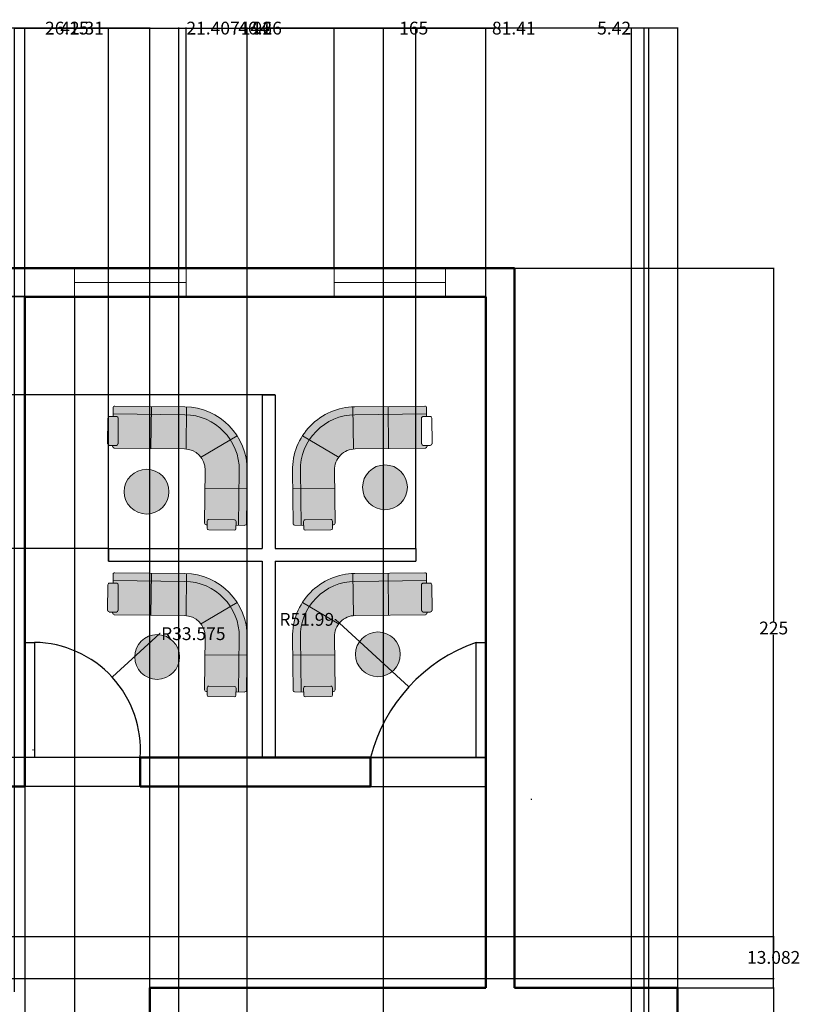
# Model space of a CAD drawing. Units: inches. Extents: x 1454 to 2136, y 626 to 1213.
# Tile 23 of 23: x 1887 to 2131, y 905 to 1213. Entities that reach past the tile are written whole.
import ezdxf

# ---------------------------------------------------------------- set-up
doc = ezdxf.new("R2010")
doc.units = ezdxf.units.IN
doc.header["$MEASUREMENT"] = 0
for name, color, linetype, lineweight in [('A-ANNO-DIMS', 2, 'Continuous', 18), ('A-DOOR', 3, 'Continuous', 25), ('A-FURN', 9, 'Continuous', 18), ('A-FURN-PATT', 252, 'Continuous', 13), ('A-FURN-PNLS', 8, 'Continuous', 25), ('A-GLAZ', 4, 'Continuous', 18), ('A-WALL', 7, 'Continuous', 50), ('sofa', 4, 'Continuous', 18)]:
    doc.layers.add(name, color=color, linetype=linetype, lineweight=lineweight)
doc.styles.get("Standard").update_dxf_attribs({"font": 'arial.ttf'})
doc.dimstyles.get("Standard").update_dxf_attribs({"dimtxt": 4, "dimasz": 0.18, "dimexe": 0.18, "dimexo": 0.0625, "dimgap": 0.09, "dimtad": 0, "dimtih": 1, "dimtoh": 1, "dimdec": 0, "dimrnd": 6, "dimzin": 0, "dimdsep": 46, "dimlunit": 3, "dimtxsty": 'Standard', "dimcen": 0.09, "dimadec": 0, "dimazin": 0, "dimtfac": 1, "dimtdec": 0, "dimtofl": 0, "dimtmove": 0, "dimatfit": 3, "dimfxl": 1, "dimtolj": 1, "dimtzin": 0, "dimarcsym": 0})

# ---------------------------------------------------------------- blocks, each defined once
blk = doc.blocks.new('A$C42183DBB')
for p, q in [((0.144, 1.661), (0.144, 1.562)), ((0.166, 1.682), (0.518, 1.682)), ((0.54, 1.661), (0.54, 1.562)), ((0, 1.592), (0, 0.864)), ((0.022, 1.614), (0.144, 1.614)), ((0.108, 1.614), (0.108, 0.864)), ((0.166, 1.541), (0.518, 1.541)), ((0.54, 1.614), (0.554, 1.614)), ((0.576, 1.592), (0.576, 0.864)), ((0, 1.11), (0.576, 1.11)), ((0.643, 0.69), (0.142, 0.389)), ((0.84, 0.576), (0.84, 0)), ((0.864, 0.576), (1.826, 0.576)), ((1.322, 0.576), (1.322, 0)), ((1.895, 0.54), (1.797, 0.54)), ((1.848, 0.54), (1.848, 0.554)), ((1.775, 0.166), (1.775, 0.518)), ((1.917, 0.166), (1.917, 0.518)), ((1.895, 0.144), (1.797, 0.144)), ((1.848, 0.022), (1.848, 0.144)), ((0.864, 0.108), (1.848, 0.108)), ((0.864, 0), (1.826, 0))]:
    blk.add_line(p, q)
for centre, radius, start, end in [((0.166, 1.661), 0.0216, 90, 180), ((0.518, 1.661), 0.0216, 0, 90), ((0.022, 1.592), 0.0216, 90, 180), ((0.166, 1.562), 0.0216, 180, 270), ((0.518, 1.562), 0.0216, 270, 0), ((0.554, 1.592), 0.0216, 0, 90), ((0.864, 0.864), 0.864, 180, 270), ((0.864, 0.864), 0.756, 180, 270), ((0.864, 0.864), 0.288, 180, 270), ((1.797, 0.518), 0.0216, 90, 180), ((1.826, 0.554), 0.0216, 0, 90), ((1.895, 0.518), 0.0216, 0, 90), ((1.797, 0.166), 0.0216, 180, 270), ((1.895, 0.166), 0.0216, 270, 0), ((1.826, 0.022), 0.0216, 270, 0)]:
    blk.add_arc(centre, radius, start, end)
blk = doc.blocks.new('WIN-34_84')
blk.add_line((34.84, 4.31), (0, 4.31))
blk.add_lwpolyline([(34.84, 0), (0, 0), (0, 9), (34.84, 9)], close=True)
blk = doc.blocks.new('DOOR-LEAF-36')
blk.add_lwpolyline([(-36, 3), (0, 3), (0, 0), (-36, 0)], close=True)
blk = doc.blocks.new('*D32')
at = {"layer": 'A-ANNO-DIMS', "color": 0, "lineweight": -2, "transparency": 16777216}
for p, q in [((1888.56, 1126.34), (1888.56, 1210.46)), ((1888.74, 1210.28), (1956.24, 1210.28)), ((2032.38, 1210.28), (1964.87, 1210.28)), ((2032.56, 1126.34), (2032.56, 1210.46))]:
    blk.add_line(p, q, dxfattribs=at)
at = {"layer": 'A-ANNO-DIMS', "color": 0, "transparency": 16777216}
for points in [[(1888.74, 1210.31), (1888.74, 1210.25), (1888.56, 1210.28)], [(2032.38, 1210.31), (2032.38, 1210.25), (2032.56, 1210.28)]]:
    blk.add_solid(points, dxfattribs=at)
at = {"layer": 'Defpoints', "color": 0, "transparency": 16777216}
for p in [(2032.56, 1210.28), (1888.56, 1126.28), (2032.56, 1126.28)]:
    blk.add_point(p, dxfattribs=at)
at = {"layer": 'A-ANNO-DIMS', "color": 0, "transparency": 16777216, "insert": (1960.56, 1210.28), "char_height": 4, "attachment_point": 5}
blk.add_mtext('\\A1;144', dxfattribs=at)
blk = doc.blocks.new('*D33')
at = {"layer": 'A-ANNO-DIMS', "color": 0, "lineweight": -2, "transparency": 16777216}
for p, q in [((2032.49, 1126.28), (1462.37, 1126.28)), ((1462.55, 1126.1), (1462.55, 1056.38)), ((1462.55, 982.46), (1462.55, 1052.18)), ((2032.49, 982.28), (1462.37, 982.28))]:
    blk.add_line(p, q, dxfattribs=at)
at = {"layer": 'A-ANNO-DIMS', "color": 0, "transparency": 16777216}
for points in [[(1462.52, 1126.1), (1462.58, 1126.1), (1462.55, 1126.28)], [(1462.52, 982.46), (1462.58, 982.46), (1462.55, 982.28)]]:
    blk.add_solid(points, dxfattribs=at)
at = {"layer": 'Defpoints', "color": 0, "transparency": 16777216}
for p in [(1462.55, 1126.28), (2032.56, 1126.28), (2032.56, 982.28)]:
    blk.add_point(p, dxfattribs=at)
at = {"layer": 'A-ANNO-DIMS', "color": 0, "transparency": 16777216, "insert": (1462.55, 1054.28), "char_height": 4, "attachment_point": 5}
blk.add_mtext('\\A1;144', dxfattribs=at)
blk = doc.blocks.new('*D34')
at = {"layer": 'A-ANNO-DIMS', "color": 0, "lineweight": -2, "transparency": 16777216}
for p, q in [((2041.62, 1135.28), (2122.74, 1135.28)), ((2122.56, 1135.1), (2122.56, 1024.91)), ((2122.56, 910.46), (2122.56, 1020.65)), ((2041.62, 910.28), (2122.74, 910.28))]:
    blk.add_line(p, q, dxfattribs=at)
at = {"layer": 'A-ANNO-DIMS', "color": 0, "transparency": 16777216}
for points in [[(2122.53, 1135.1), (2122.59, 1135.1), (2122.56, 1135.28)], [(2122.53, 910.46), (2122.59, 910.46), (2122.56, 910.28)]]:
    blk.add_solid(points, dxfattribs=at)
at = {"layer": 'Defpoints', "color": 0, "transparency": 16777216}
for p in [(2041.56, 1135.28), (2041.56, 910.28), (2122.56, 910.28)]:
    blk.add_point(p, dxfattribs=at)
at = {"layer": 'A-ANNO-DIMS', "color": 0, "transparency": 16777216, "insert": (2122.56, 1022.78), "char_height": 4, "attachment_point": 5}
blk.add_mtext('\\A1;225', dxfattribs=at)
blk = doc.blocks.new('*D35')
at = {"layer": 'A-ANNO-DIMS', "color": 0, "lineweight": -2, "transparency": 16777216}
for p, q in [((2092.62, 910.28), (2122.74, 910.28)), ((2122.56, 910.1), (2122.56, 808.91)), ((2122.56, 703.46), (2122.56, 804.65)), ((2092.62, 703.28), (2122.74, 703.28))]:
    blk.add_line(p, q, dxfattribs=at)
at = {"layer": 'A-ANNO-DIMS', "color": 0, "transparency": 16777216}
for points in [[(2122.53, 910.1), (2122.59, 910.1), (2122.56, 910.28)], [(2122.53, 703.46), (2122.59, 703.46), (2122.56, 703.28)]]:
    blk.add_solid(points, dxfattribs=at)
at = {"layer": 'Defpoints', "color": 0, "transparency": 16777216}
for p in [(2092.56, 910.28), (2092.56, 703.28), (2122.56, 703.28)]:
    blk.add_point(p, dxfattribs=at)
at = {"layer": 'A-ANNO-DIMS', "color": 0, "transparency": 16777216, "insert": (2122.56, 806.78), "char_height": 4, "attachment_point": 5}
blk.add_mtext('\\A1;207', dxfattribs=at)
blk = doc.blocks.new('*D36')
at = {"layer": 'A-ANNO-DIMS', "color": 0, "lineweight": -2, "transparency": 16777216}
for p, q in [((1927.56, 910.34), (1927.56, 1210.46)), ((1927.74, 1210.28), (2005.72, 1210.28)), ((2092.38, 1210.28), (2014.39, 1210.28)), ((2092.56, 910.34), (2092.56, 1210.46))]:
    blk.add_line(p, q, dxfattribs=at)
at = {"layer": 'A-ANNO-DIMS', "color": 0, "transparency": 16777216}
for points in [[(1927.74, 1210.31), (1927.74, 1210.25), (1927.56, 1210.28)], [(2092.38, 1210.31), (2092.38, 1210.25), (2092.56, 1210.28)]]:
    blk.add_solid(points, dxfattribs=at)
at = {"layer": 'Defpoints', "color": 0, "transparency": 16777216}
for p in [(2092.56, 1210.28), (1927.56, 910.28), (2092.56, 910.28)]:
    blk.add_point(p, dxfattribs=at)
at = {"layer": 'A-ANNO-DIMS', "color": 0, "transparency": 16777216, "insert": (2010.06, 1210.28), "char_height": 4, "attachment_point": 5}
blk.add_mtext('\\A1;165', dxfattribs=at)
blk = doc.blocks.new('*D37')
at = {"layer": 'A-ANNO-DIMS', "color": 0, "lineweight": -2, "transparency": 16777216}
for p, q in [((1774.56, 712.34), (1774.56, 1210.46)), ((1774.74, 1210.28), (1846.74, 1210.28)), ((1927.38, 1210.28), (1855.38, 1210.28)), ((1927.56, 712.34), (1927.56, 1210.46))]:
    blk.add_line(p, q, dxfattribs=at)
at = {"layer": 'A-ANNO-DIMS', "color": 0, "transparency": 16777216}
for points in [[(1774.74, 1210.31), (1774.74, 1210.25), (1774.56, 1210.28)], [(1927.38, 1210.31), (1927.38, 1210.25), (1927.56, 1210.28)]]:
    blk.add_solid(points, dxfattribs=at)
at = {"layer": 'Defpoints', "color": 0, "transparency": 16777216}
for p in [(1927.56, 1210.28), (1774.56, 712.28), (1927.56, 712.28)]:
    blk.add_point(p, dxfattribs=at)
at = {"layer": 'A-ANNO-DIMS', "color": 0, "transparency": 16777216, "insert": (1851.06, 1210.28), "char_height": 4, "attachment_point": 5}
blk.add_mtext('\\A1;153', dxfattribs=at)
blk = doc.blocks.new('*D47')
at = {"layer": 'A-ANNO-DIMS', "color": 0, "lineweight": -2, "transparency": 16777216}
for p, q in [((1885.25, 909.11), (1885.25, 1210.46)), ((1885.43, 1210.28), (1899.87, 1210.28)), ((1927.38, 1210.28), (1912.94, 1210.28)), ((1927.56, 910.34), (1927.56, 1210.46))]:
    blk.add_line(p, q, dxfattribs=at)
at = {"layer": 'A-ANNO-DIMS', "color": 0, "transparency": 16777216}
for points in [[(1885.43, 1210.31), (1885.43, 1210.25), (1885.25, 1210.28)], [(1927.38, 1210.31), (1927.38, 1210.25), (1927.56, 1210.28)]]:
    blk.add_solid(points, dxfattribs=at)
at = {"layer": 'Defpoints', "color": 0, "transparency": 16777216}
for p in [(1885.25, 1210.28), (1885.25, 909.05), (1927.56, 910.28)]:
    blk.add_point(p, dxfattribs=at)
at = {"layer": 'A-ANNO-DIMS', "color": 0, "transparency": 16777216, "insert": (1906.4, 1210.28), "char_height": 4, "attachment_point": 5}
blk.add_mtext('\\A1;42.31', dxfattribs=at)
blk = doc.blocks.new('*D58')
at = {"layer": 'A-ANNO-DIMS', "color": 0, "lineweight": -2, "transparency": 16777216}
for p, q in [((1654.43, 926.36), (2122.74, 926.36)), ((2122.56, 926.18), (2122.56, 921.96)), ((2122.56, 913.46), (2122.56, 917.69)), ((1654.62, 913.28), (2122.74, 913.28))]:
    blk.add_line(p, q, dxfattribs=at)
at = {"layer": 'A-ANNO-DIMS', "color": 0, "transparency": 16777216}
for points in [[(2122.53, 926.18), (2122.59, 926.18), (2122.56, 926.36)], [(2122.53, 913.46), (2122.59, 913.46), (2122.56, 913.28)]]:
    blk.add_solid(points, dxfattribs=at)
at = {"layer": 'Defpoints', "color": 0, "transparency": 16777216}
for p in [(1654.37, 926.36), (2122.56, 926.36), (1654.56, 913.28)]:
    blk.add_point(p, dxfattribs=at)
at = {"layer": 'A-ANNO-DIMS', "color": 0, "transparency": 16777216, "insert": (2122.56, 919.82), "char_height": 4, "attachment_point": 5}
blk.add_mtext('\\A1;13.082', dxfattribs=at)
blk = doc.blocks.new('*D61')
at = {"layer": 'A-ANNO-DIMS', "color": 0, "lineweight": -2, "transparency": 16777216}
for p, q in [((1904.06, 1126.38), (1904.06, 628.1)), ((1888.56, 1126.22), (1888.56, 628.1)), ((1888.74, 628.28), (1903.88, 628.28)), ((1904.06, 628.28), (1904.24, 628.28))]:
    blk.add_line(p, q, dxfattribs=at)
at = {"layer": 'A-ANNO-DIMS', "color": 0, "transparency": 16777216}
for points in [[(1888.74, 628.31), (1888.74, 628.25), (1888.56, 628.28)], [(1903.88, 628.31), (1903.88, 628.25), (1904.06, 628.28)]]:
    blk.add_solid(points, dxfattribs=at)
at = {"layer": 'Defpoints', "color": 0, "transparency": 16777216}
for p in [(1904.06, 1126.44), (1888.56, 1126.28), (1904.06, 628.28)]:
    blk.add_point(p, dxfattribs=at)
at = {"layer": 'A-ANNO-DIMS', "color": 0, "transparency": 16777216, "insert": (1912.45, 628.28), "char_height": 4, "attachment_point": 5}
blk.add_mtext('\\A1;15.506', dxfattribs=at)
blk = doc.blocks.new('*D62')
at = {"layer": 'A-ANNO-DIMS', "color": 0, "lineweight": -2, "transparency": 16777216}
for p, q in [((1938.9, 1135.5), (1938.9, 1210.46)), ((1939.08, 1210.28), (1955.11, 1210.28)), ((1984.98, 1210.28), (1968.95, 1210.28)), ((1985.16, 1135.5), (1985.16, 1210.46))]:
    blk.add_line(p, q, dxfattribs=at)
at = {"layer": 'A-ANNO-DIMS', "color": 0, "transparency": 16777216}
for points in [[(1939.08, 1210.31), (1939.08, 1210.25), (1938.9, 1210.28)], [(1984.98, 1210.31), (1984.98, 1210.25), (1985.16, 1210.28)]]:
    blk.add_solid(points, dxfattribs=at)
at = {"layer": 'Defpoints', "color": 0, "transparency": 16777216}
for p in [(1985.16, 1210.28), (1938.9, 1135.44), (1985.16, 1135.44)]:
    blk.add_point(p, dxfattribs=at)
at = {"layer": 'A-ANNO-DIMS', "color": 0, "transparency": 16777216, "insert": (1962.03, 1210.28), "char_height": 4, "attachment_point": 5}
blk.add_mtext('\\A1;46.26', dxfattribs=at)
blk = doc.blocks.new('*D63')
at = {"layer": 'A-ANNO-DIMS', "color": 0, "lineweight": -2, "transparency": 16777216}
for p, q in [((2000.63, 733.98), (2000.63, 1210.46)), ((2000.81, 1210.28), (2034.88, 1210.28)), ((2081.86, 1210.28), (2047.79, 1210.28)), ((2082.04, 733.98), (2082.04, 1210.46))]:
    blk.add_line(p, q, dxfattribs=at)
at = {"layer": 'A-ANNO-DIMS', "color": 0, "transparency": 16777216}
for points in [[(2000.81, 1210.31), (2000.81, 1210.25), (2000.63, 1210.28)], [(2081.86, 1210.31), (2081.86, 1210.25), (2082.04, 1210.28)]]:
    blk.add_solid(points, dxfattribs=at)
at = {"layer": 'Defpoints', "color": 0, "transparency": 16777216}
for p in [(2082.04, 1210.28), (2000.63, 733.92), (2082.04, 733.92)]:
    blk.add_point(p, dxfattribs=at)
at = {"layer": 'A-ANNO-DIMS', "color": 0, "transparency": 16777216, "insert": (2041.33, 1210.28), "char_height": 4, "attachment_point": 5}
blk.add_mtext('\\A1;81.41', dxfattribs=at)
blk = doc.blocks.new('*D73')
at = {"layer": 'A-ANNO-DIMS', "color": 0, "lineweight": -2, "transparency": 16777216}
for p, q in [((1985.1, 1126.44), (1462.37, 1126.44)), ((1462.55, 1126.26), (1462.55, 1113.18)), ((1462.55, 1095.83), (1462.55, 1108.91)), ((1966.64, 1095.65), (1462.37, 1095.65))]:
    blk.add_line(p, q, dxfattribs=at)
at = {"layer": 'A-ANNO-DIMS', "color": 0, "transparency": 16777216}
for points in [[(1462.52, 1126.26), (1462.58, 1126.26), (1462.55, 1126.44)], [(1462.52, 1095.83), (1462.58, 1095.83), (1462.55, 1095.65)]]:
    blk.add_solid(points, dxfattribs=at)
at = {"layer": 'Defpoints', "color": 0, "transparency": 16777216}
for p in [(1985.16, 1126.44), (1462.55, 1095.65), (1966.71, 1095.65)]:
    blk.add_point(p, dxfattribs=at)
at = {"layer": 'A-ANNO-DIMS', "color": 0, "transparency": 16777216, "insert": (1462.55, 1111.04), "char_height": 4, "attachment_point": 5}
blk.add_mtext('\\A1;30.79', dxfattribs=at)
blk = doc.blocks.new('*D74')
at = {"layer": 'A-ANNO-DIMS', "color": 0, "lineweight": -2, "transparency": 16777216}
for p, q in [((1888.56, 1018.34), (1888.56, 1210.46)), ((1888.74, 1210.28), (1894.74, 1210.28)), ((1914.53, 1210.28), (1908.52, 1210.28)), ((1914.71, 1043.71), (1914.71, 1210.46))]:
    blk.add_line(p, q, dxfattribs=at)
at = {"layer": 'A-ANNO-DIMS', "color": 0, "transparency": 16777216}
for points in [[(1888.74, 1210.31), (1888.74, 1210.25), (1888.56, 1210.28)], [(1914.53, 1210.31), (1914.53, 1210.25), (1914.71, 1210.28)]]:
    blk.add_solid(points, dxfattribs=at)
at = {"layer": 'Defpoints', "color": 0, "transparency": 16777216}
for p in [(1914.71, 1210.28), (1914.71, 1043.65), (1888.56, 1018.28)]:
    blk.add_point(p, dxfattribs=at)
at = {"layer": 'A-ANNO-DIMS', "color": 0, "transparency": 16777216, "insert": (1901.63, 1210.28), "char_height": 4, "attachment_point": 5}
blk.add_mtext('\\A1;26.15', dxfattribs=at)
blk = doc.blocks.new('*D75')
at = {"layer": 'A-ANNO-DIMS', "color": 0, "lineweight": -2, "transparency": 16777216}
for p, q in [((1914.71, 1047.71), (1914.71, 1210.46)), ((1914.89, 1210.28), (1959.75, 1210.28)), ((2010.53, 1210.28), (1965.66, 1210.28)), ((2010.71, 1047.71), (2010.71, 1210.46))]:
    blk.add_line(p, q, dxfattribs=at)
at = {"layer": 'A-ANNO-DIMS', "color": 0, "transparency": 16777216}
for points in [[(1914.89, 1210.31), (1914.89, 1210.25), (1914.71, 1210.28)], [(2010.53, 1210.31), (2010.53, 1210.25), (2010.71, 1210.28)]]:
    blk.add_solid(points, dxfattribs=at)
at = {"layer": 'Defpoints', "color": 0, "transparency": 16777216}
for p in [(2010.71, 1210.28), (1914.71, 1047.65), (2010.71, 1047.65)]:
    blk.add_point(p, dxfattribs=at)
at = {"layer": 'A-ANNO-DIMS', "color": 0, "transparency": 16777216, "insert": (1962.71, 1210.28), "char_height": 4, "attachment_point": 5}
blk.add_mtext('\\A1;96', dxfattribs=at)
blk = doc.blocks.new('*D76')
at = {"layer": 'A-ANNO-DIMS', "color": 0, "lineweight": -2, "transparency": 16777216}
for p, q in [((1962.64, 1095.65), (1462.37, 1095.65)), ((1462.55, 1095.47), (1462.55, 1073.78)), ((1462.55, 1047.83), (1462.55, 1069.52)), ((1914.64, 1047.65), (1462.37, 1047.65))]:
    blk.add_line(p, q, dxfattribs=at)
at = {"layer": 'A-ANNO-DIMS', "color": 0, "transparency": 16777216}
for points in [[(1462.52, 1095.47), (1462.58, 1095.47), (1462.55, 1095.65)], [(1462.52, 1047.83), (1462.58, 1047.83), (1462.55, 1047.65)]]:
    blk.add_solid(points, dxfattribs=at)
at = {"layer": 'Defpoints', "color": 0, "transparency": 16777216}
for p in [(1962.71, 1095.65), (1462.55, 1047.65), (1914.71, 1047.65)]:
    blk.add_point(p, dxfattribs=at)
at = {"layer": 'A-ANNO-DIMS', "color": 0, "transparency": 16777216, "insert": (1462.55, 1071.65), "char_height": 4, "attachment_point": 5}
blk.add_mtext('\\A1;48', dxfattribs=at)
blk = doc.blocks.new('*D83')
at = {"layer": 'A-ANNO-DIMS', "color": 0, "lineweight": -2, "transparency": 16777216}
for p, q in [((1936.64, 835.68), (1936.64, 1210.46)), ((1936.82, 1210.28), (1938.91, 1210.28)), ((1957.86, 1210.28), (1955.77, 1210.28)), ((1958.04, 828.71), (1958.04, 1210.46))]:
    blk.add_line(p, q, dxfattribs=at)
at = {"layer": 'A-ANNO-DIMS', "color": 0, "transparency": 16777216}
for points in [[(1936.82, 1210.31), (1936.82, 1210.25), (1936.64, 1210.28)], [(1957.86, 1210.31), (1957.86, 1210.25), (1958.04, 1210.28)]]:
    blk.add_solid(points, dxfattribs=at)
at = {"layer": 'Defpoints', "color": 0, "transparency": 16777216}
for p in [(1958.04, 1210.28), (1936.64, 835.61), (1958.04, 828.64)]:
    blk.add_point(p, dxfattribs=at)
at = {"layer": 'A-ANNO-DIMS', "color": 0, "transparency": 16777216, "insert": (1947.34, 1210.28), "char_height": 4, "attachment_point": 5}
blk.add_mtext('\\A1;21.407', dxfattribs=at)
blk = doc.blocks.new('*D86')
at = {"layer": 'A-ANNO-DIMS', "color": 0, "lineweight": -2, "transparency": 16777216}
for p, q in [((2078.14, 1210.28), (2077.96, 1210.28)), ((2078.14, 776.98), (2078.14, 1210.46)), ((2083.38, 1210.28), (2078.32, 1210.28)), ((2083.56, 712.34), (2083.56, 1210.46))]:
    blk.add_line(p, q, dxfattribs=at)
at = {"layer": 'A-ANNO-DIMS', "color": 0, "transparency": 16777216}
for points in [[(2078.32, 1210.31), (2078.32, 1210.25), (2078.14, 1210.28)], [(2083.38, 1210.31), (2083.38, 1210.25), (2083.56, 1210.28)]]:
    blk.add_solid(points, dxfattribs=at)
at = {"layer": 'Defpoints', "color": 0, "transparency": 16777216}
for p in [(2078.14, 1210.28), (2078.14, 776.92), (2083.56, 712.28)]:
    blk.add_point(p, dxfattribs=at)
at = {"layer": 'A-ANNO-DIMS', "color": 0, "transparency": 16777216, "insert": (2072.69, 1210.28), "char_height": 4, "attachment_point": 5}
blk.add_mtext('\\A1;5.42', dxfattribs=at)
blk = doc.blocks.new('*D90')
at = {"layer": 'A-ANNO-DIMS', "color": 0, "lineweight": -2, "transparency": 16777216}
for p, q in [((1985.39, 1025.48), (1985.57, 1025.48)), ((1985.57, 1025.48), (2008.43, 1004.52)), ((2046.8, 969.26), (2046.98, 969.26)), ((2046.89, 969.17), (2046.89, 969.35))]:
    blk.add_line(p, q, dxfattribs=at)
at = {"layer": 'A-ANNO-DIMS', "color": 0, "transparency": 16777216}
blk.add_solid([(2008.45, 1004.54), (2008.41, 1004.5), (2008.57, 1004.4)], dxfattribs=at)
at = {"layer": 'Defpoints', "color": 0, "transparency": 16777216}
for p in [(2008.57, 1004.4), (2046.89, 969.26)]:
    blk.add_point(p, dxfattribs=at)
at = {"layer": 'A-ANNO-DIMS', "color": 0, "transparency": 16777216, "insert": (1976.63, 1025.48), "char_height": 4, "attachment_point": 5}
blk.add_mtext('\\A1;R51.99', dxfattribs=at)
blk = doc.blocks.new('*D97')
at = {"layer": 'A-ANNO-DIMS', "color": 0, "lineweight": -2, "transparency": 16777216}
for p, q in [((1930.67, 1021.01), (1915.95, 1007.52)), ((1930.85, 1021.01), (1930.67, 1021.01)), ((1891.07, 984.62), (1891.07, 984.8)), ((1890.98, 984.71), (1891.16, 984.71))]:
    blk.add_line(p, q, dxfattribs=at)
at = {"layer": 'A-ANNO-DIMS', "color": 0, "transparency": 16777216}
blk.add_solid([(1915.93, 1007.54), (1915.97, 1007.5), (1915.82, 1007.4)], dxfattribs=at)
at = {"layer": 'Defpoints', "color": 0, "transparency": 16777216}
for p in [(1915.82, 1007.4), (1891.07, 984.71)]:
    blk.add_point(p, dxfattribs=at)
at = {"layer": 'A-ANNO-DIMS', "color": 0, "transparency": 16777216, "insert": (1941.17, 1021.01), "char_height": 4, "attachment_point": 5}
blk.add_mtext('\\A1;R33.575', dxfattribs=at)

msp = doc.modelspace()

# ---------------------------------------------------------------- hatches: boundary and pattern name
at = {"layer": 'A-FURN-PATT'}
h = msp.add_hatch(dxfattribs=at)
h.set_pattern_fill('ESCHER', color=256)
h.paths.add_polyline_path([(1511.3761, 923.7174, 1), (1525.379, 923.7174, 1)])
h.paths.add_polyline_path([(1525.379, 816.0542, 1), (1511.3761, 816.0542, 1)])
h.paths.add_polyline_path([(1525.379, 712.7345, 1), (1511.3761, 712.7345, 1)])
h.paths.add_polyline_path([(2070.5057, 794.3402, 1), (2056.5027, 794.3402, 1)])
h.paths.add_polyline_path([(2005.868, 1014.5578, 1), (1991.8651, 1014.5578, 1)])
h.paths.add_polyline_path([(1994.0647, 1066.7584, 1), (2008.0677, 1066.7584, 1)])
h.paths.add_polyline_path([(1919.5492, 1065.3848, 1), (1933.5521, 1065.3848, 1)])
h.paths.add_polyline_path([(1936.8517, 1013.7336, 1), (1922.8488, 1013.7336, 1)])
h.paths.add_polyline_path([(1824.6062, 1109.1557, 1), (1838.6091, 1109.1557, 1)])
h = msp.add_hatch(color=256, dxfattribs=at)
h.dxf.hatch_style = 1
h.paths.add_polyline_path([(1855.0231, 1089.5248, 0.41421356), (1850.0231, 1094.5248), (1811.2288, 1094.5248, 0.41421356), (1806.2288, 1089.5248), (1806.2288, 1083.6305, 0.41421356), (1811.2288, 1078.6305), (1850.0231, 1078.6305, 0.41421356), (1855.0231, 1083.6305)])
h.paths.add_polyline_path([(1939.0638, 1089.4209), (1938.9354, 1078.7354, -0.20858653), (1943.5258, 1076.1857), (1952.7682, 1081.5837, 0.24238954)])
h.paths.add_polyline_path([(1939.0638, 1089.4209, 0.00796483), (1938.5148, 1089.4363), (1928.0643, 1089.5619), (1927.936, 1078.8906), (1938.3866, 1078.765, -0.02092855), (1938.9354, 1078.7354)])
h.paths.add_polyline_path([(1928.0643, 1089.5619), (1916.0797, 1089.706), (1916.0698, 1088.8851), (1917.241, 1088.8711, -0.41420041), (1917.7276, 1088.3726), (1917.6308, 1080.3281, -0.41422672), (1917.1324, 1079.8415), (1915.9612, 1079.8556), (1915.9573, 1079.5272, 0.41420799), (1916.4439, 1079.0288), (1927.936, 1078.8906)])
h.paths.add_polyline_path([(1917.7276, 1088.3726, 0.41420041), (1917.241, 1088.8711), (1914.9926, 1088.8981, 0.41421356), (1914.4941, 1088.4115), (1914.3974, 1080.367, 0.41421356), (1914.884, 1079.8686), (1917.1324, 1079.8415, 0.41422672), (1917.6308, 1080.3281)])
h.paths.add_polyline_path([(1928.0939, 1092.0245), (1916.6018, 1092.1627, 0.41422672), (1916.1033, 1091.6761), (1916.0797, 1089.706), (1928.0643, 1089.5619)])
h.paths.add_polyline_path([(1939.0935, 1091.8846, 0.00696804), (1938.5445, 1091.8989), (1928.0939, 1092.0245), (1928.0643, 1089.5619), (1938.5148, 1089.4363, -0.00796483), (1939.0638, 1089.4209)])
h.paths.add_polyline_path([(1939.0935, 1091.8846), (1939.0638, 1089.4209, -0.24238954), (1952.7682, 1081.5837), (1954.897, 1082.827, 0.24500473)])
h.paths.add_polyline_path([(1952.7682, 1081.5837), (1943.5258, 1076.1857, -0.16768112), (1944.8746, 1072.1191), (1944.8073, 1066.5201), (1955.4785, 1066.3918), (1955.5459, 1071.9909, 0.14799784)])
h.paths.add_polyline_path([(1954.897, 1082.827), (1952.7682, 1081.5837, -0.14799784), (1955.5459, 1071.9909), (1955.4785, 1066.3918), (1957.9412, 1066.3622), (1958.0085, 1071.9612, 0.14649407)])
h.paths.add_polyline_path([(1955.4785, 1066.3918), (1944.8073, 1066.5201), (1944.675, 1055.5205, 0.41421356), (1945.1616, 1055.0221), (1945.49, 1055.0181), (1945.5041, 1056.1893, -0.41421356), (1946.0025, 1056.6759), (1954.047, 1056.5792, -0.41421356), (1954.5336, 1056.0807), (1954.5195, 1054.9096), (1955.3404, 1054.8997)])
h.paths.add_polyline_path([(1954.5336, 1056.0807, 0.41421356), (1954.047, 1056.5792), (1946.0025, 1056.6759, 0.41421356), (1945.5041, 1056.1893), (1945.49, 1055.0181), (1945.477, 1053.9409, 0.41422115), (1945.9636, 1053.4425), (1954.0081, 1053.3458, 0.41420598), (1954.5066, 1053.8324)])
h.paths.add_polyline_path([(1957.9412, 1066.3622), (1955.4785, 1066.3918), (1955.3404, 1054.8997), (1957.3105, 1054.876, 0.41421356), (1957.8089, 1055.3626)])
h.paths.add_polyline_path([(1974.6911, 1066.3918), (1972.2285, 1066.3622), (1972.3608, 1055.3626, 0.41421356), (1972.8592, 1054.876), (1974.8293, 1054.8997)])
h.paths.add_polyline_path([(1985.3624, 1066.5201), (1974.6911, 1066.3918), (1974.8293, 1054.8997), (1975.6501, 1054.9096), (1975.6361, 1056.0807, -0.41421356), (1976.1227, 1056.5792), (1984.1672, 1056.6759, -0.41421356), (1984.6656, 1056.1893), (1984.6797, 1055.0181), (1985.008, 1055.0221, 0.41421356), (1985.4946, 1055.5205)])
h.paths.add_polyline_path([(1984.6656, 1056.1893, 0.41421356), (1984.1672, 1056.6759), (1976.1227, 1056.5792, 0.41421356), (1975.6361, 1056.0807), (1975.6631, 1053.8324, 0.41422115), (1976.1615, 1053.3458), (1984.206, 1053.4425, 0.41420597), (1984.6926, 1053.9409)])
h.paths.add_polyline_path([(1985.2951, 1072.1191, -0.16768112), (1986.6438, 1076.1857), (1977.4014, 1081.5837, 0.14799988), (1974.6238, 1071.9907), (1974.6911, 1066.3918), (1985.3624, 1066.5201)])
h.paths.add_polyline_path([(1977.4014, 1081.5837), (1975.2727, 1082.827, 0.14649407), (1972.1612, 1071.9612), (1972.2285, 1066.3622), (1974.6911, 1066.3918), (1974.6238, 1071.9907, -0.14799988)])
h.paths.add_polyline_path([(1991.1058, 1089.4209, 0.24238954), (1977.4014, 1081.5837), (1986.6438, 1076.1857, -0.20858653), (1991.2343, 1078.7354)])
h.paths.add_polyline_path([(1991.1058, 1089.4209), (1991.0762, 1091.8846, 0.24500473), (1975.2727, 1082.827), (1977.4014, 1081.5837, -0.24238954)])
h.paths.add_polyline_path([(2002.1053, 1089.5619), (1991.6547, 1089.4363, 0.00796283), (1991.1058, 1089.4209), (1991.2343, 1078.7354, -0.02092855), (1991.783, 1078.765), (2002.2336, 1078.8906)])
h.paths.add_polyline_path([(2002.0757, 1092.0245), (1991.6251, 1091.8989, 0.00696804), (1991.0762, 1091.8846), (1991.1058, 1089.4209, -0.00796283), (1991.6547, 1089.4363), (2002.1053, 1089.5619)])
h.paths.add_polyline_path([(2014.0663, 1091.6761, 0.4142004), (2013.5679, 1092.1627), (2002.0757, 1092.0245), (2002.1053, 1089.5619), (2014.09, 1089.706)])
h.paths.add_polyline_path([(2012.4421, 1088.3726, -0.41422672), (2012.9287, 1088.8711), (2014.0999, 1088.8851), (2014.09, 1089.706), (2002.1053, 1089.5619), (2002.2336, 1078.8906), (2013.7258, 1079.0288, 0.41421913), (2014.2124, 1079.5273), (2014.2084, 1079.8556), (2013.0373, 1079.8415, -0.4142004), (2012.5388, 1080.3281)])
h.paths.add_polyline_path([(1986.6438, 1024.0964), (1977.4014, 1029.4944, 0.14799988), (1974.6238, 1019.9014), (1974.6911, 1014.3025), (1985.3624, 1014.4308), (1985.2951, 1020.0298, -0.16768112)])
h.paths.add_polyline_path([(1991.1058, 1037.3316, 0.24238954), (1977.4014, 1029.4944), (1986.6438, 1024.0964, -0.20858653), (1991.2343, 1026.6461)])
h.paths.add_polyline_path([(2002.1053, 1037.4726), (1991.6547, 1037.347, 0.00796283), (1991.1058, 1037.3316), (1991.2343, 1026.6461, -0.02092855), (1991.783, 1026.6757), (2002.2336, 1026.8013)])
h.paths.add_polyline_path([(2012.4421, 1036.2833, -0.41422672), (2012.9287, 1036.7818), (2014.0999, 1036.7958), (2014.09, 1037.6167), (2002.1053, 1037.4726), (2002.2336, 1026.8013), (2013.7258, 1026.9395, 0.41421913), (2014.2124, 1027.438), (2014.2084, 1027.7663), (2013.0373, 1027.7522, -0.4142004), (2012.5388, 1028.2388)])
h.paths.add_polyline_path([(2015.6755, 1036.3222, 0.41421356), (2015.1771, 1036.8088), (2012.9287, 1036.7818, 0.41422672), (2012.4421, 1036.2833), (2012.5388, 1028.2388, 0.4142004), (2013.0373, 1027.7522), (2015.2856, 1027.7793, 0.41421356), (2015.7722, 1028.2777)])
h.paths.add_polyline_path([(1985.3624, 1014.4308), (1974.6911, 1014.3025), (1974.8293, 1002.8104), (1975.6501, 1002.8203), (1975.6361, 1003.9914, -0.41421356), (1976.1227, 1004.4899), (1984.1672, 1004.5866, -0.41421356), (1984.6656, 1004.1), (1984.6797, 1002.9288), (1985.008, 1002.9328, 0.41421356), (1985.4946, 1003.4312)])
h.paths.add_polyline_path([(1984.6656, 1004.1, 0.41421356), (1984.1672, 1004.5866), (1976.1227, 1004.4899, 0.41421356), (1975.6361, 1003.9914), (1975.6631, 1001.743, 0.41422115), (1976.1615, 1001.2564), (1984.206, 1001.3532, 0.41420598), (1984.6926, 1001.8516)])
h.paths.add_polyline_path([(1974.6911, 1014.3025), (1972.2285, 1014.2729), (1972.3608, 1003.2733, 0.41421356), (1972.8592, 1002.7867), (1974.8293, 1002.8104)])
h.paths.add_polyline_path([(1974.6238, 1019.9014, -0.14799988), (1977.4014, 1029.4944), (1975.2727, 1030.7376, 0.14649407), (1972.1612, 1019.8719), (1972.2285, 1014.2729), (1974.6911, 1014.3025)])
h.paths.add_polyline_path([(1991.1058, 1037.3316), (1991.0762, 1039.7953, 0.24500473), (1975.2727, 1030.7376), (1977.4014, 1029.4944, -0.24238954)])
h.paths.add_polyline_path([(2002.0757, 1039.9352), (1991.6251, 1039.8096, 0.00696804), (1991.0762, 1039.7953), (1991.1058, 1037.3316, -0.00796283), (1991.6547, 1037.347), (2002.1053, 1037.4726)])
h.paths.add_polyline_path([(2014.0663, 1039.5868, 0.4142004), (2013.5679, 1040.0734), (2002.0757, 1039.9352), (2002.1053, 1037.4726), (2014.09, 1037.6167)])
h.paths.add_polyline_path([(1955.5459, 1019.9016, 0.14799784), (1952.7682, 1029.4944), (1943.5258, 1024.0964, -0.16768112), (1944.8746, 1020.0298), (1944.8073, 1014.4308), (1955.4785, 1014.3025)])
h.paths.add_polyline_path([(1955.4785, 1014.3025), (1944.8073, 1014.4308), (1944.675, 1003.4312, 0.41421356), (1945.1616, 1002.9328), (1945.49, 1002.9288), (1945.5041, 1004.1, -0.41421356), (1946.0025, 1004.5866), (1954.047, 1004.4899, -0.41421356), (1954.5336, 1003.9914), (1954.5195, 1002.8203), (1955.3404, 1002.8104)])
h.paths.add_polyline_path([(1939.0638, 1037.3316), (1938.9354, 1026.6461, -0.20858653), (1943.5258, 1024.0964), (1952.7682, 1029.4944, 0.24238954)])
h.paths.add_polyline_path([(1939.0638, 1037.3316, 0.00796483), (1938.5148, 1037.347), (1928.0643, 1037.4726), (1927.936, 1026.8013), (1938.3866, 1026.6757, -0.02092855), (1938.9354, 1026.6461)])
h.paths.add_polyline_path([(1928.0643, 1037.4726), (1916.0797, 1037.6167), (1916.0698, 1036.7958), (1917.241, 1036.7818, -0.41420041), (1917.7276, 1036.2833), (1917.6308, 1028.2388, -0.41422672), (1917.1324, 1027.7522), (1915.9612, 1027.7663), (1915.9573, 1027.4379, 0.41420799), (1916.4439, 1026.9395), (1927.936, 1026.8013)])
h.paths.add_polyline_path([(1917.7276, 1036.2833, 0.41420041), (1917.241, 1036.7818), (1914.9926, 1036.8088, 0.41421356), (1914.4941, 1036.3222), (1914.3974, 1028.2777, 0.41421356), (1914.884, 1027.7793), (1917.1324, 1027.7522, 0.41422672), (1917.6308, 1028.2388)])
h.paths.add_polyline_path([(1928.0939, 1039.9352), (1916.6018, 1040.0734, 0.41422672), (1916.1033, 1039.5868), (1916.0797, 1037.6167), (1928.0643, 1037.4726)])
h.paths.add_polyline_path([(1939.0935, 1039.7953, 0.00696804), (1938.5445, 1039.8096), (1928.0939, 1039.9352), (1928.0643, 1037.4726), (1938.5148, 1037.347, -0.00796483), (1939.0638, 1037.3316)])
h.paths.add_polyline_path([(1939.0935, 1039.7953), (1939.0638, 1037.3316, -0.24238954), (1952.7682, 1029.4944), (1954.897, 1030.7376, 0.24500473)])
h.paths.add_polyline_path([(1954.897, 1030.7376), (1952.7682, 1029.4944, -0.14799784), (1955.5459, 1019.9016), (1955.4785, 1014.3025), (1957.9412, 1014.2729), (1958.0085, 1019.8719, 0.14649407)])
h.paths.add_polyline_path([(1957.9412, 1014.2729), (1955.4785, 1014.3025), (1955.3404, 1002.8104), (1957.3105, 1002.7867, 0.41421356), (1957.8089, 1003.2733)])
h.paths.add_polyline_path([(1954.5336, 1003.9914, 0.41421356), (1954.047, 1004.4899), (1946.0025, 1004.5866, 0.41421356), (1945.5041, 1004.1), (1945.49, 1002.9288), (1945.477, 1001.8516, 0.41422115), (1945.9636, 1001.3532), (1954.0081, 1001.2564, 0.41420598), (1954.5066, 1001.743)])
h.paths.add_polyline_path([(1997.553, 886.9384), (1981.0334, 886.9384), (1981.0334, 876.3409, 0.41421356), (1984.1503, 873.224), (1996.6179, 873.224, 0.41421356), (1999.7348, 876.3409), (1998.488, 876.3409, -0.41421356), (1997.553, 877.276)])
h.paths.add_polyline_path([(1981.0334, 886.9384), (1964.5139, 886.9384), (1964.5139, 877.276, -0.41421356), (1963.5788, 876.3409), (1962.3321, 876.3409, 0.41421356), (1965.449, 873.224), (1977.9165, 873.224, 0.41421356), (1981.0334, 876.3409)])
h.paths.add_polyline_path([(1964.5139, 886.9384), (1964.5139, 887.25, 0.47353022), (1963.4209, 888.1978, -0.46345458), (1962.3321, 889.1202), (1962.3321, 890.6786), (1962.3321, 892.5488), (1961.0853, 892.5488, 0.41421356), (1960.1503, 891.6137), (1960.1503, 877.276, 0.41421356), (1961.0853, 876.3409), (1963.5788, 876.3409, 0.41421356), (1964.5139, 877.276)])
h.paths.add_polyline_path([(1999.7348, 892.5488), (1999.7348, 893.7955, 0.41421356), (1998.7997, 894.7306), (1963.2672, 894.7306, 0.41421356), (1962.3321, 893.7955), (1962.3321, 892.5488), (1962.3321, 890.3669, 0.41421356), (1963.2672, 889.4319), (1998.7997, 889.4319, 0.41421356), (1999.7348, 890.3669), (1999.7348, 890.6786)])
h.paths.add_polyline_path([(2001.9166, 891.6137, 0.41421356), (2000.9815, 892.5488), (1999.7348, 892.5488), (1999.7348, 890.6786), (1999.7348, 890.3669), (1999.7348, 889.1202, -0.41421356), (1998.7997, 888.1851), (1998.488, 888.1851, 0.41421356), (1997.553, 887.25), (1997.553, 877.276, 0.41421356), (1998.488, 876.3409), (1999.7348, 876.3409), (2000.9815, 876.3409, 0.41421356), (2001.9166, 877.276)])
h.paths.add_polyline_path([(1999.7348, 889.1202), (1999.7348, 890.3669, -0.41421356), (1998.7997, 889.4319), (1963.2672, 889.4319, -0.41421356), (1962.3321, 890.3669), (1962.3321, 889.1202, 0.46345458), (1963.4209, 888.1978, -0.45647258), (1964.5139, 887.3025), (1964.5139, 886.9384), (1997.553, 886.9384), (1997.553, 887.25, -0.41421356), (1998.488, 888.1851), (1998.7997, 888.1851, 0.41421356)])
h.paths.add_polyline_path([(1540.5701, 966.1379, 0.41421356), (1538.9915, 967.7165), (1523.2061, 967.7165, 0.41421356), (1521.6275, 966.1379), (1521.6275, 964.5679, 0.41579661), (1523.2061, 962.9808), (1538.9915, 962.9808, 0.41421356), (1540.5701, 964.5594)])
h.paths.add_polyline_path([(1538.9151, 960.1995, 0.41421356), (1537.968, 961.1466), (1524.2565, 961.1466, 0.41421356), (1523.3094, 960.1995), (1523.3094, 947.859, 0.41421356), (1524.2565, 946.9119), (1537.968, 946.9119, 0.41421356), (1538.9151, 947.859)])
h.paths.add_polyline_path([(1555.8609, 960.5704, 0.41421356), (1554.9138, 961.5176), (1543.8299, 961.5176, 0.41421356), (1542.8828, 960.5704), (1542.8828, 946.859, 0.41421356), (1543.8299, 945.9119), (1554.9138, 945.9119, 0.41421356), (1555.8609, 946.859)])
h.paths.add_polyline_path([(1555.8609, 941.6364, 0.41421356), (1554.9138, 942.5835), (1543.8299, 942.5835, 0.41421356), (1542.8828, 941.6364), (1542.8828, 927.9249, 0.41421356), (1543.8299, 926.9778), (1554.9138, 926.9778, 0.41421356), (1555.8609, 927.9249)])
h.paths.add_polyline_path([(1555.8609, 922.6938, 0.41421356), (1554.9138, 923.6409), (1543.8299, 923.6409, 0.41421356), (1542.8828, 922.6938), (1542.8828, 908.9824, 0.41421356), (1543.8299, 908.0352), (1554.9138, 908.0352, 0.41421356), (1555.8609, 908.9824)])
h.paths.add_polyline_path([(1555.8609, 815.2921, 0.41421356), (1554.9138, 816.2392), (1543.8299, 816.2392, 0.41421356), (1542.8828, 815.2921), (1542.8828, 801.5806, 0.41421356), (1543.8299, 800.6335), (1554.9138, 800.6335, 0.41421356), (1555.8609, 801.5806)])
h.paths.add_polyline_path([(1555.8609, 834.2346, 0.41421356), (1554.9138, 835.1818), (1543.8299, 835.1818, 0.41421356), (1542.8828, 834.2346), (1542.8828, 820.5232, 0.41421356), (1543.8299, 819.576), (1554.9138, 819.576, 0.41421356), (1555.8609, 820.5232)])
h.paths.add_polyline_path([(1555.8609, 853.1687, 0.41421356), (1554.9138, 854.1158), (1543.8299, 854.1158, 0.41421356), (1542.8828, 853.1687), (1542.8828, 839.4572, 0.41421356), (1543.8299, 838.5101), (1554.9138, 838.5101, 0.41421356), (1555.8609, 839.4572)])
h.paths.add_polyline_path([(1538.9151, 852.7977, 0.41421356), (1537.968, 853.7448), (1524.2565, 853.7448, 0.41421356), (1523.3094, 852.7977), (1523.3094, 840.4573, 0.41421356), (1524.2565, 839.5101), (1537.968, 839.5101, 0.41421356), (1538.9151, 840.4573)])
h.paths.add_polyline_path([(1538.9151, 748.5053, 0.41421356), (1537.968, 749.4524), (1524.2565, 749.4524, 0.41421356), (1523.3094, 748.5053), (1523.3094, 736.1648, 0.41421356), (1524.2565, 735.2177), (1537.968, 735.2177, 0.41421356), (1538.9151, 736.1648)])
h.paths.add_polyline_path([(1555.8609, 748.8763, 0.41421356), (1554.9138, 749.8234), (1543.8299, 749.8234, 0.41421356), (1542.8828, 748.8763), (1542.8828, 735.1648, 0.41421356), (1543.8299, 734.2177), (1554.9138, 734.2177, 0.41421356), (1555.8609, 735.1648)])
h.paths.add_polyline_path([(1555.8609, 729.9422, 0.41421356), (1554.9138, 730.8893), (1543.8299, 730.8893, 0.41421356), (1542.8828, 729.9422), (1542.8828, 716.2308, 0.41421356), (1543.8299, 715.2836), (1554.9138, 715.2836, 0.41421356), (1555.8609, 716.2308)])
h.paths.add_polyline_path([(1555.8609, 710.9996, 0.41421356), (1554.9138, 711.9468), (1543.8299, 711.9468, 0.41421356), (1542.8828, 710.9996), (1542.8828, 697.2882, 0.41421356), (1543.8299, 696.3411), (1554.9138, 696.3411, 0.41421356), (1555.8609, 697.2882)])
h.paths.add_polyline_path([(1562.4308, 712.0232, 0.44500955), (1560.6884, 713.5932), (1559.1098, 713.5932, 0.3840739), (1557.6951, 712.0232), (1557.6951, 696.2377, 0.43158582), (1559.3667, 694.6619), (1560.9452, 694.6619, 0.39705211), (1562.4308, 696.2377)])
h.paths.add_polyline_path([(1559.2737, 713.6017, -0.41421356), (1557.6951, 715.1803), (1557.6951, 730.9658, -0.39284205), (1559.1577, 732.5401, -0.39284205), (1557.6951, 734.1143), (1557.6951, 749.8998, -0.41421356), (1559.2737, 751.4784), (1560.8522, 751.4784, -0.41421356), (1562.4308, 749.8998), (1562.4308, 734.1143, -0.39284205), (1560.9682, 732.5401, -0.39284205), (1562.4308, 730.9658), (1562.4308, 715.1803, -0.41421356), (1560.8522, 713.6017), (1559.2737, 713.5932), (1559.4375, 713.5932, 0.05204098), (1559.1098, 713.5932)])
h.paths.add_polyline_path([(1559.2737, 732.5443), (1559.2737, 732.5358), (1560.8522, 732.5358), (1560.8522, 732.5443)], flags=16)
h.paths.add_polyline_path([(1562.4308, 749.8998, 0.41421356), (1560.8522, 751.4784), (1559.2737, 751.4784, 0.41421356), (1557.6951, 749.8998), (1557.6951, 734.1143, 0.41421356), (1559.2737, 732.5358), (1559.2737, 732.5443, 0.41421356), (1557.6951, 730.9658), (1557.6951, 715.1803, 0.41421356), (1559.2737, 713.6017), (1560.8437, 713.6018, 0.41579661), (1562.4308, 715.1803), (1562.4308, 730.9658, 0.41421356), (1560.8522, 732.5443), (1560.8522, 732.5358, 0.41421356), (1562.4308, 734.1143)])

# ---------------------------------------------------------------- linework, layer by layer
at = {"layer": 'A-DOOR'}
for p, q in [((1924.5563, 982.2825), (1888.5563, 982.2825)), ((1996.5563, 982.2825), (2032.5563, 982.2825)), ((1924.5563, 973.2825), (1888.5563, 973.2825)), ((1996.5563, 973.2825), (2032.5563, 973.2825))]:
    msp.add_line(p, q, dxfattribs=at)
for centre, radius, start, end in [((1891.0693, 984.711), 33.5749, 355.851988, 89.168906), ((2046.8936, 969.2649), 51.9932, 109.478468, 165.500638)]:
    msp.add_arc(centre, radius, start, end, dxfattribs=at)
at = {"layer": 'A-FURN'}
for centre in [(1926.5506, 1065.3848), (2001.0662, 1066.7584), (1929.8503, 1013.7336), (1998.8666, 1014.5578)]:
    msp.add_circle(centre, 7.0015, dxfattribs=at)
at = {"layer": 'A-FURN-PNLS'}
for p, q in [((1962.7068, 1095.6495), (1962.7068, 1047.6495)), ((1962.7068, 1095.6495), (1966.7068, 1095.6495)), ((1966.7068, 1095.6495), (1966.7068, 1047.6495)), ((1914.7068, 1047.6495), (1962.7068, 1047.6495)), ((1914.7068, 1047.6495), (1914.7068, 1043.6495)), ((1966.7068, 1047.6495), (2010.7068, 1047.6495)), ((2010.7068, 1047.6495), (2010.7068, 1043.6495)), ((1914.7068, 1043.6495), (1962.7068, 1043.6495)), ((1962.7068, 1043.6495), (1962.7068, 982.2825)), ((1966.7068, 1043.6495), (2010.7068, 1043.6495)), ((1966.7068, 1043.6495), (1966.7068, 982.2825))]:
    msp.add_line(p, q, dxfattribs=at)
at = {"layer": 'A-WALL'}
for p, q in [((2041.5563, 1135.2825), (1759.5563, 1135.2825)), ((2041.5563, 1135.2825), (2041.5563, 910.2825)), ((2032.5563, 1126.2825), (1888.5563, 1126.2825)), ((1888.5563, 1126.2825), (1888.5563, 973.2825)), ((2032.5563, 1126.2825), (2032.5563, 910.2825)), ((1996.5563, 982.2825), (1924.5563, 982.2825)), ((1924.5563, 982.2825), (1924.5563, 973.2825)), ((1996.5563, 982.2825), (1996.5563, 973.2825)), ((1888.5563, 973.2825), (1879.5563, 973.2825)), ((1996.5563, 973.2825), (1924.5563, 973.2825)), ((1927.5563, 784.2825), (1927.5563, 910.2825)), ((2032.5563, 910.2825), (1927.5563, 910.2825)), ((2092.5563, 910.2825), (2041.5563, 910.2825)), ((2092.5563, 703.2825), (2092.5563, 910.2825))]:
    msp.add_line(p, q, dxfattribs=at)

# ---------------------------------------------------------------- block references
at = {"layer": 'A-DOOR', "rotation": 90.00000000000033}
for p in [(1891.5563, 1018.2825), (2032.5563, 1018.2825)]:
    msp.add_blockref('DOOR-LEAF-36', p, dxfattribs=at)
at = {"layer": 'A-GLAZ'}
for p in [(1904.0619, 1126.439), (1985.158, 1126.439)]:
    msp.add_blockref('WIN-34_84', p, dxfattribs=at)
at = {"layer": 'sofa', "yscale": 22.80350778510874, "zscale": 22.80350778510874}
for p, xscale, rotation in [((1958.2453, 1091.662), 22.80350778510874, 179.3111670300788), ((1971.9243, 1091.662), -22.80350778510874, 180.6888329699211), ((1958.2453, 1039.5727), 22.80350778510874, 179.3111670300788), ((1971.9243, 1039.5727), -22.80350778510874, 180.6888329699211)]:
    msp.add_blockref('A$C42183DBB', p, dxfattribs=dict(at, xscale=xscale, rotation=rotation))

# ---------------------------------------------------------------- dimensions: what is measured, and where the dimension line sits
at = {"layer": 'A-ANNO-DIMS'}
for base, p1, p2, override, picture, middle in [((1927.5563, 1210.2845), (1774.5563, 712.2825), (1927.5563, 712.2825), {"dimdec": 0, "dimlfac": 1, "dimrnd": 0, "dimzin": 0, "dimdsep": 46, "dimlunit": 2}, '*D37', (1851.0563, 1210.2845)), ((1885.2497, 1210.2845), (1927.5563, 910.2825), (1885.2497, 909.0476), {"dimdec": 2, "dimlfac": 1, "dimrnd": 0, "dimzin": 0, "dimdsep": 46, "dimlunit": 2}, '*D47', (1906.403, 1210.2845)), ((2032.5563, 1210.2845), (1888.5563, 1126.2825), (2032.5563, 1126.2825), {"dimdec": 0, "dimlfac": 1, "dimrnd": 0, "dimzin": 0, "dimdsep": 46, "dimlunit": 2}, '*D32', (1960.5563, 1210.2845)), ((1914.7068, 1210.2845), (1888.5563, 1018.2825), (1914.7068, 1043.6495), {"dimdec": 2, "dimlfac": 1, "dimrnd": 0, "dimzin": 0, "dimdsep": 46, "dimlunit": 2}, '*D74', (1901.6316, 1210.2845)), ((2010.7068, 1210.2845), (1914.7068, 1047.6495), (2010.7068, 1047.6495), {"dimdec": 0, "dimlfac": 1, "dimrnd": 0, "dimzin": 0, "dimdsep": 46, "dimlunit": 2}, '*D75', (1962.7068, 1210.2845)), ((2092.5563, 1210.2845), (1927.5563, 910.2825), (2092.5563, 910.2825), {"dimdec": 0, "dimlfac": 1, "dimrnd": 0, "dimzin": 0, "dimdsep": 46, "dimlunit": 2}, '*D36', (2010.0563, 1210.2845)), ((1958.0422, 1210.2845), (1936.6352, 835.6136), (1958.0422, 828.6443), {"dimdec": 3, "dimlfac": 1, "dimrnd": 0, "dimzin": 0, "dimdsep": 46, "dimlunit": 2}, '*D83', (1947.3387, 1210.2845)), ((1985.158, 1210.2845), (1938.9022, 1135.439), (1985.158, 1135.439), {"dimdec": 2, "dimlfac": 1, "dimrnd": 0, "dimzin": 0, "dimdsep": 46, "dimlunit": 2}, '*D62', (1962.0301, 1210.2845)), ((2082.0362, 1210.2845), (2000.6276, 733.9205), (2082.0362, 733.9205), {"dimdec": 2, "dimlfac": 1, "dimrnd": 0, "dimzin": 0, "dimdsep": 46, "dimlunit": 2}, '*D63', (2041.3319, 1210.2845)), ((2078.1364, 1210.2845), (2083.5563, 712.2825), (2078.1364, 776.9179), {"dimdec": 2, "dimlfac": 1, "dimrnd": 0, "dimzin": 0, "dimdsep": 46, "dimlunit": 2}, '*D86', (2072.6917, 1210.2845)), ((1904.0619, 628.2805), (1888.5563, 1126.2825), (1904.0619, 1126.439), {"dimdec": 3, "dimlfac": 1, "dimrnd": 0, "dimzin": 0, "dimdsep": 46, "dimlunit": 2}, '*D61', (1912.4452, 628.2805))]:
    dim = msp.add_linear_dim(base=base, p1=p1, p2=p2, dimstyle='Standard', override=override, dxfattribs=at)
    dim.commit()
    dim.dimension.update_dxf_attribs({"geometry": picture, "text_midpoint": middle})
for base, p1, p2, override, picture, middle in [((2122.5583, 910.2825), (2041.5563, 1135.2825), (2041.5563, 910.2825), {"dimdec": 0, "dimlfac": 1, "dimrnd": 0, "dimzin": 0, "dimdsep": 46, "dimlunit": 2}, '*D34', (2122.5583, 1022.7825)), ((1462.5543, 1095.6495), (1985.158, 1126.439), (1966.7068, 1095.6495), {"dimdec": 2, "dimlfac": 1, "dimrnd": 0, "dimzin": 0, "dimdsep": 46, "dimlunit": 2}, '*D73', (1462.5543, 1111.0443)), ((1462.5543, 1126.2825), (2032.5563, 982.2825), (2032.5563, 1126.2825), {"dimdec": 0, "dimlfac": 1, "dimrnd": 0, "dimzin": 0, "dimdsep": 46, "dimlunit": 2}, '*D33', (1462.5543, 1054.2825)), ((1462.5543, 1047.6495), (1962.7068, 1095.6495), (1914.7068, 1047.6495), {"dimdec": 0, "dimlfac": 1, "dimrnd": 0, "dimzin": 0, "dimdsep": 46, "dimlunit": 2}, '*D76', (1462.5543, 1071.6495)), ((2122.55832, 926.36405), (1654.55632, 913.28246), (1654.37233, 926.36405), {"dimdec": 3, "dimlfac": 1, "dimrnd": 0, "dimzin": 0, "dimdsep": 46, "dimlunit": 2}, '*D58', (2122.55832, 919.82325)), ((2122.5583, 703.2825), (2092.5563, 910.2825), (2092.5563, 703.2825), {"dimdec": 0, "dimlfac": 1, "dimrnd": 0, "dimzin": 0, "dimdsep": 46, "dimlunit": 2}, '*D35', (2122.5583, 806.7825))]:
    dim = msp.add_linear_dim(base=base, p1=p1, p2=p2, angle=90, dimstyle='Standard', override=override, dxfattribs=at)
    dim.commit()
    dim.dimension.update_dxf_attribs({"geometry": picture, "text_midpoint": middle})
for center, mpoint, override, picture, middle in [((2046.8936, 969.2649), (2008.5667, 1004.3982), {"dimdec": 2, "dimlfac": 1, "dimrnd": 0, "dimzin": 0, "dimdsep": 46, "dimlunit": 2}, '*D90', (1976.6335, 1025.4782)), ((1891.0693, 984.711), (1915.8194, 1007.3983), {"dimdec": 3, "dimlfac": 1, "dimrnd": 0, "dimzin": 0, "dimdsep": 46, "dimlunit": 2}, '*D97', (1941.1713, 1021.0107))]:
    dim = msp.add_radius_dim(center=center, mpoint=mpoint, dimstyle='Standard', override=override, dxfattribs=at)
    dim.commit()
    dim.dimension.update_dxf_attribs({"geometry": picture, "text_midpoint": middle, "dimtype": 164})

doc.saveas('drawing.dxf')
